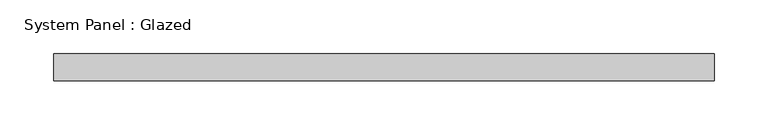
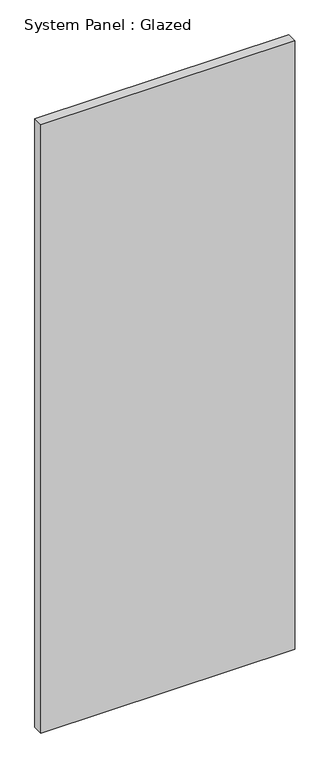
"""IFC4 building model written with IfcOpenShell, lengths in millimetres: plate geometry, System Panel : Glazed."""

from ifc_helpers import new_model, si_unit, origin, origin_with_axes, place, context, project, spatial, polyline, outline, extrude, source, transform, mapped, element, save


def system_panel_glazed_2519712b(model_context):
    return source(origin(), model_context, "Body", "SweptSolid", [
        extrude(outline(polyline([(307.975, 19.05), (-307.975, 19.05), (-307.975, 44.45), (307.975, 44.45), (307.975, 19.05)])), origin_with_axes(), (0.0, 0.0, 1.0), 1560.096911),
    ])


if __name__ == "__main__":
    model = new_model("IFC4")
    model_context = context("Model", 3, world=origin())
    ifc_project = project(units=[si_unit("LENGTHUNIT", "METRE", prefix="MILLI")], contexts=[model_context])
    site = spatial("IfcSite", under=ifc_project)
    building = spatial("IfcBuilding", under=site)
    placement = place(None, origin())
    system_panel_glazed_shape = system_panel_glazed_2519712b(model_context)
    element("IfcPlate", 1, ObjectType="System Panel : Glazed", at=placement, inside=building, context=model_context, shape_type="MappedRepresentation", body=[
        mapped(system_panel_glazed_shape, transform((0.0, 0.0, 0.0), x_axis=(1.0, 0.0, 0.0), y_axis=(0.0, 1.0, 0.0), z_axis=(0.0, 0.0, 1.0))),
    ])
    save(model, "model.ifc")

# Revit data of these elements
# Type "System Panel : Glazed"
#   Construction Type Id = "GSP4R"
#   Analytic Construction = "1/8 in Pilkington single glazing"
#   Visual Light Transmittance = 0.9
#   Solar Heat Gain Coefficient = 0.86
#   Heat Transfer Coefficient (U) = 1.18115 BTU/(h·ft²·°F)
#   Define Thermal Properties by = 1
# Element 1 (IfcPlate, "System Panel : Glazed")
#   Materials on its faces: "Glass"
# Materials
#   "Glass": class "Glass", colour RGB 0 128 192, transparency 0.75, Description = "Soda Lime Glass", Cost = 0
